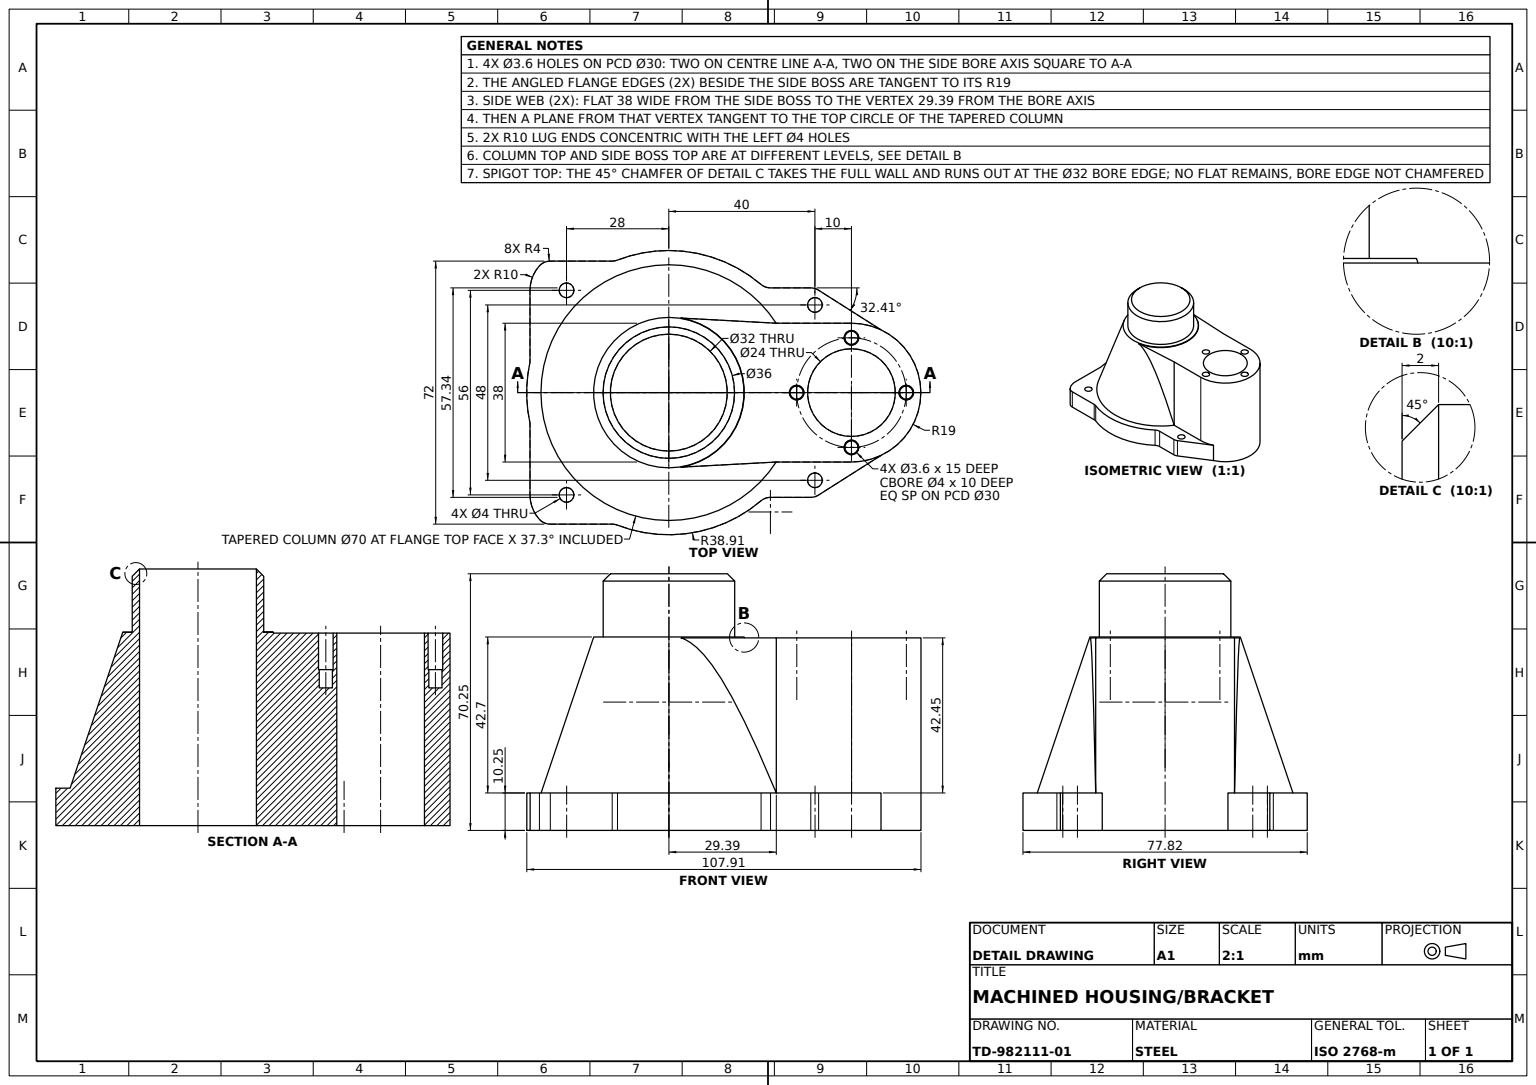
SolidWorks part; units mm, degrees
material "Plain Carbon Steel"
ref_plane "Front Plane" through (0, 0, 0) normal (0, 0, 1) x (1, 0, 0)
ref_plane "Top Plane" through (0, 0, 0) normal (0, 1, 0) x (1, 0, 0)
ref_plane "Right Plane" through (0, 0, 0) normal (1, 0, 0) x (0, 0, -1)
sketch "Base Flange Sketch" plane through (0, 0, 0) normal (0, 1, 0) x (1, 0, 0)
  line L1 (40.9814, 28.048) -> (58.0582, 17.2066)
  line L2 (38.8375, 28.6711) -> (27.8179, 28.6711)
  line L3 (40.9814, -28.048) -> (58.0582, -17.2066)
  line L5 (38.8375, -28.6711) -> (27.8179, -28.6711)
  line L7 (-28, 36) -> (-15.5318, 36)
  line L10 (-38, -28) -> (-38, -8.3642)
  line L12 (-38, 28) -> (-38, 8.3642)
  line L13 (-38, -28) -> (-38, -8.3642)
  line L15 (-28, 36) -> (-32.4721, 36)
  line L16 (-28, -36) -> (-32.4721, -36)
  line L17 (-28, -36) -> (-15.5318, -36)
  arc A0 (58.0582, -17.2066) -> (58.0582, 17.2066) centre (50, 0) ccw
  arc A2 (-14.0839, -36.2712) -> (25.2248, -29.6255) centre (0, 0) ccw
  arc A3 (-38, -28) -> (-35.4536, -34.6667) centre (-28, -28) ccw
  arc A4 (25.2248, 29.6255) -> (-14.0839, 36.2712) centre (0, 0) ccw
  arc A5 (-19.2177, 32.7823) -> (-19.6886, 33.5607) centre (-28, 28) ccw
  arc A6 (-35.4536, 34.6667) -> (-38, 28) centre (-28, 28) ccw
  arc A8 (-34, -36) -> (-38, -28) centre (-28, -28) cw
  arc A9 (-38, 8.3642) -> (-38, -8.3642) centre (0, 0) ccw
  arc A10 (38.8375, -28.6711) -> (40.9814, -28.048) centre (38.8375, -24.6711) ccw
  arc A11 (40.9814, 28.048) -> (38.8375, 28.6711) centre (38.8375, 24.6711) ccw
  arc A12 (27.8179, 28.6711) -> (25.2248, 29.6255) centre (27.8179, 32.6711) cw
  arc A13 (-15.5318, -36) -> (-14.0839, -36.2712) centre (-15.5318, -40) cw
  arc A14 (-15.5318, 36) -> (-14.0839, 36.2712) centre (-15.5318, 40) ccw
  arc A15 (27.8179, -28.6711) -> (25.2248, -29.6255) centre (27.8179, -32.6711) ccw
  arc A16 (-35.4536, -34.6667) -> (-32.4721, -36) centre (-32.4721, -32) ccw
  arc A17 (-32.4721, 36) -> (-35.4536, 34.6667) centre (-32.4721, 32) ccw
  point P40 (-34, 36)
  dimension "D1" = 4
  dimension "D2" = 4
  dimension "D3" = 19
  dimension "D4" = 38.9096
  dimension "D5" = 10
  dimension "D6" = 4
  dimension "D7" = 2.5464
  dimension "D8" = 18.3114
  dimension "D9" = 22.4682
  dimension "D10" = 63.2248
  dimension "D11" = 18.7823
  dimension "D12" = 76.8375
  dimension "D13" = 78.9814
  dimension "D14" = 88
extrude "Base Flange" add sketch "Base Flange Sketch" along normal blind 10.25
sketch "Tapered Column Sketch" plane through (0, 10.25, 0) normal (0, 1, 0) x (1, 0, 0)
  circle A0 centre (0, 0) radius 35
  dimension "D1" = 70
ref_plane "Plane1" through (0, 42.85, 0) normal (0, 1, 0) x (1, 0, 0)
extrude "Tapered Column" add sketch "Tapered Column Sketch" along normal blind 42.7 draft 18.65
sketch "Top Boss Sketch" plane through (0, 52.95, 0) normal (0, 1, 0) x (1, 0, 0)
  circle A0 centre (0, 0) radius 18
  dimension "D1" = 36
extrude "Top Boss" add sketch "Top Boss Sketch" along normal blind 15.3
sketch "Top Collar Sketch" plane through (0, 68.25, 0) normal (0, 1, 0) x (1, 0, 0)
  circle A0 centre (0, 0) radius 18
  dimension "D1" = 36
extrude "Top Collar 45deg Taper" add sketch "Top Collar Sketch" along normal blind 2 draft 45
sketch "Side Boss Sketch" plane through (0, 10.25, 0) normal (0, 1, 0) x (1, 0, 0)
  line L0 (50, 19) -> (29.3939, 19)
  line L1 (50, -19) -> (29.3939, -19)
  line L2 (29.3939, 19) -> (0, 20.5884)
  line L3 (29.3939, -19) -> (0, -20.5884)
  arc A0 (50, -19) -> (50, 19) centre (50, 0) ccw
  circle A1 centre (0, 0) radius 35 construction
  circle A3 centre (0, 0) radius 20.5884 construction
  arc A4 (0, 20.5884) -> (0, -20.5884) centre (0, 0) cw
  circle M5 centre (0, 0) radius 35
  arc M21 (58.0582, -17.2066) -> (58.0582, 17.2066) centre (50, 0) ccw
  dimension "D1" = 19
extrude "Side Boss" add sketch "Side Boss Sketch" along normal blind 42.45 contours L1 A0 L0 M21 M5 | L2 A4 L3 M5
sketch "Side Boss Holes Sketch" plane through (0, 52.7, 0) normal (0, 1, 0) x (1, 0, 0)
  circle A1 centre (35, 0) radius 2
  circle A2 centre (50, 15) radius 2
  circle A3 centre (65, 0) radius 2
  circle A4 centre (50, -15) radius 2
  dimension "D1" = 4
  dimension "D2" = 4
  dimension "D3" = 15
  dimension "D4" = 4
extrude "Side Boss Holes 4x Depth 10" cut sketch "Side Boss Holes Sketch" against normal blind 10
sketch "Secondary Holes Sketch" plane through (0, 42.7, 0) normal (0, 1, 0) x (1, 0, 0)
  circle A0 centre (35, 0) radius 1.8
  circle A1 centre (65, 0) radius 1.8
  circle A2 centre (50, -15) radius 1.8
  circle A3 centre (50, 15) radius 1.8
  dimension "D1" = 3.6
extrude "Secondary Holes 4x Depth 5" cut sketch "Secondary Holes Sketch" against normal blind 5
sketch "Side Bore Sketch" plane through (0, 52.7, 0) normal (0, 1, 0) x (1, 0, 0)
  circle A0 centre (50, 0) radius 12
  dimension "D1" = 24
extrude "Side Bore" cut sketch "Side Bore Sketch" against normal blind 177
sketch "Main Bore Sketch" plane through (0, 70.25, 0) normal (0, 1, 0) x (1, 0, 0)
  circle A0 centre (0, 0) radius 16
  dimension "D1" = 32
extrude "Main Bore" cut sketch "Main Bore Sketch" against normal blind 177
sketch "Flange Holes Sketch" plane through (0, 10.25, 0) normal (0, 1, 0) x (1, 0, 0)
  line L0 (50, -19) -> (29.3939, -19) construction
  circle A1 centre (40, -24) radius 2
  circle A2 centre (40, 24) radius 2
  circle A4 centre (-28, 28) radius 2
  circle A5 centre (-28, -28) radius 2
  dimension "D1" = 4
  dimension "D2" = 10
  dimension "D3" = 78
  dimension "D4" = 43
  dimension "D5" = 47
  dimension "D6" = 5
  dimension "D7" = 9
extrude "Flange Holes 4x" cut sketch "Flange Holes Sketch" against normal blind 177
